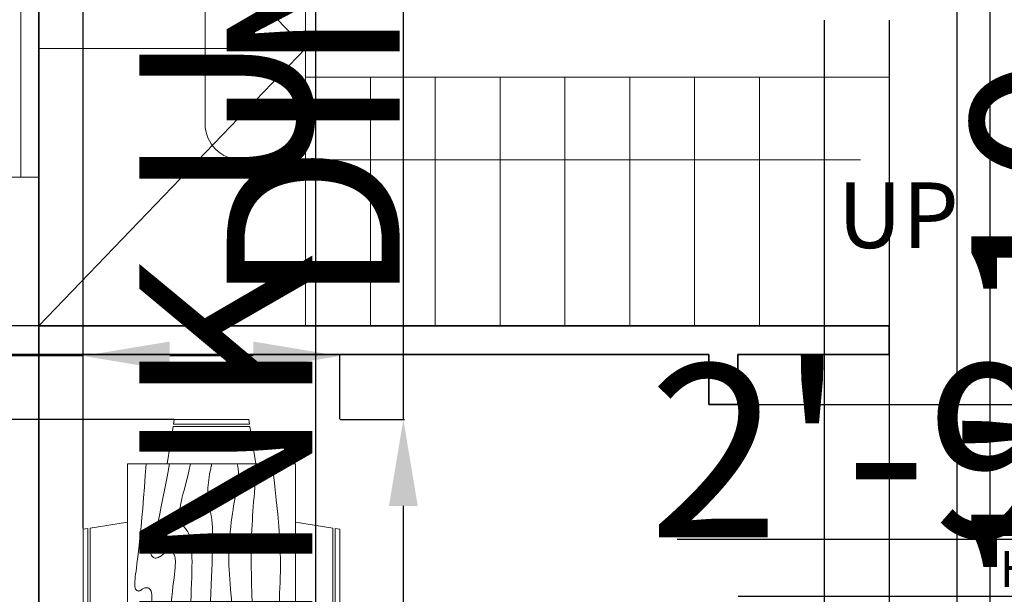
# Model space of a CAD drawing. Units: inches. Extents: x 2236 to 2927, y 1577 to 2452.
# Tile 4 of 9: x 2413 to 2550, y 1836 to 1916. Entities that reach past the tile are written whole.
import ezdxf

# ---------------------------------------------------------------- set-up
doc = ezdxf.new("R2010")
doc.units = ezdxf.units.IN
for name, color, linetype, lineweight in [('A-ANNO-DIMS', 2, 'Continuous', 18), ('A-ANNO-SYMB', 7, 'Continuous', 18), ('A-ANNO-TEXT', 7, 'Continuous', 18), ('A-AREA-IDEN', 7, 'Continuous', 18), ('A-FURN', 8, 'Continuous', 18), ('Steps', 50, 'Continuous', 18), ('Wall', 7, 'Continuous', 35), ('Windows', 162, 'Continuous', 18)]:
    doc.layers.add(name, color=color, linetype=linetype, lineweight=lineweight)
doc.styles.get("Standard").update_dxf_attribs({"font": 'arial.ttf'})
doc.dimstyles.get("Standard").update_dxf_attribs({"dimtxt": 24, "dimasz": 12, "dimexe": 0.18, "dimexo": 0.0625, "dimgap": 0.09, "dimtad": 1, "dimdec": 1, "dimzin": 0, "dimdsep": 46, "dimlunit": 4, "dimtxsty": 'Standard', "dimcen": 0.09, "dimadec": 0, "dimazin": 0, "dimtfac": 1, "dimtdec": 1, "dimtofl": 0, "dimtmove": 0, "dimatfit": 3, "dimfxl": 1, "dimtolj": 1, "dimtzin": 0, "dimarcsym": 0})

# ---------------------------------------------------------------- blocks, each defined once
blk = doc.blocks.new('Dining Set - 36 x 72 in.')
for p, q in [((-22, 27.5), (-22.1562, 26.50042)), ((-22, 27.5), (-6, 27.5)), ((-5.8437, 26.49966), (-6, 27.5)), ((6, 27.5), (5.8438, 26.50042)), ((6, 27.5), (22, 27.5)), ((22.1563, 26.49966), (22, 27.5)), ((-22.2343, 26.00059), (-23.4847, 17.99762)), ((-22.2304, 26), (-5.7608, 26)), ((-5.8416, 26.5), (-22.1534, 26.5)), ((-4.5152, 17.99762), (-5.7655, 25.99926)), ((5.7657, 26.00059), (4.5153, 17.99762)), ((5.7696, 26), (22.2392, 26)), ((22.1584, 26.5), (5.8466, 26.5)), ((23.4848, 17.99762), (22.2345, 25.99926)), ((36, 18), (-36, 18)), ((-36, 18), (-36, -18)), ((36, -18), (36, 18)), ((-44.0006, 8.23428), (-35.9976, 9.48474)), ((44.0006, 8.23428), (35.9976, 9.48474)), ((-45.5, 8), (-44.5004, 8.15617)), ((-45.5, 8), (-45.5, -8)), ((-44.5, -8.15843), (-44.5, 8.15338)), ((-44, 8.23041), (-44, -8.23915)), ((44, 8.23041), (44, -8.23915)), ((44.5, -8.15843), (44.5, 8.15338)), ((45.5, 8), (44.5005, 8.15617)), ((45.5, 8), (45.5, -8)), ((-44.4997, -8.15631), (-45.5, -8)), ((-35.9976, -9.48476), (-43.9993, -8.2345)), ((35.9976, -9.48476), (43.9993, -8.2345)), ((44.4997, -8.15631), (45.5, -8)), ((-36, -18), (36, -18)), ((-22.2343, -26.0006), (-23.4847, -17.99762)), ((-4.5152, -17.99762), (-5.7655, -25.99928)), ((5.7657, -26.0006), (4.5153, -17.99762)), ((23.4848, -17.99762), (22.2345, -25.99928)), ((-22.2304, -26), (-5.7608, -26)), ((-22, -27.5), (-22.1562, -26.50044)), ((-5.8416, -26.5), (-22.1534, -26.5)), ((-5.8437, -26.49967), (-6, -27.5)), ((5.7696, -26), (22.2392, -26)), ((6, -27.5), (5.8438, -26.50044)), ((22.1584, -26.5), (5.8466, -26.5)), ((22.1563, -26.49967), (22, -27.5)), ((-22, -27.5), (-6, -27.5)), ((6, -27.5), (22, -27.5))]:
    blk.add_line(p, q)
for points in [[(-36, 15), (-31.1772, 14.97754), (-26.8079, 14.91406), (-22.8538, 14.81543), (-19.276, 14.6875), (-16.0362, 14.53613), (-13.0957, 14.36718), (-10.4159, 14.18652), (-7.9583, 14), (-5.6904, 13.81315), (-3.6035, 13.63021), (-1.6954, 13.45508), (0.0365, 13.29166), (1.5945, 13.14388), (2.9811, 13.01562), (4.1988, 12.9108), (5.25, 12.83333), (6.1393, 12.78613), (6.8802, 12.76823), (7.4883, 12.77767), (7.9792, 12.8125), (8.3685, 12.87077), (8.6719, 12.95052), (8.9049, 13.0498), (9.0833, 13.16666), (9.2205, 13.29899), (9.3216, 13.44401), (9.3895, 13.59879), (9.4271, 13.76041), (9.4373, 13.92594), (9.4232, 14.09245), (9.3875, 14.257), (9.3333, 14.41666), (9.2638, 14.56917), (9.1836, 14.71484), (9.0975, 14.85465), (9.0104, 14.98958), (8.9272, 15.1206), (8.8529, 15.2487), (8.7922, 15.37483), (8.75, 15.5), (8.7305, 15.62467), (8.7344, 15.74739), (8.7617, 15.86621), (8.8125, 15.97916), (8.8867, 16.08431), (8.9844, 16.17968), (9.1055, 16.26334), (9.25, 16.33333), (9.4189, 16.38802), (9.6172, 16.42708), (9.8506, 16.45052), (10.125, 16.45833), (10.4463, 16.45052), (10.8203, 16.42708), (11.2529, 16.38802), (11.75, 16.33333), (12.3184, 16.26318), (12.9694, 16.17838), (13.7151, 16.07991), (14.5677, 15.96875), (15.5395, 15.84586), (16.6426, 15.71224), (17.8893, 15.56884), (19.2917, 15.41666), (20.859, 15.25667), (22.5879, 15.08984), (24.4721, 14.91715), (26.5052, 14.73958), (28.6809, 14.5581), (30.9929, 14.3737), (33.4347, 14.18733), (36, 14)], [(-36, 10), (-28.9766, 10.14274), (-23.1725, 10.20442), (-18.4241, 10.19775), (-14.5677, 10.13541), (-11.4399, 10.03011), (-8.877, 9.89453), (-6.7154, 9.74137), (-4.7917, 9.58333), (-2.9698, 9.43082), (-1.2246, 9.28515), (0.4415, 9.14534), (2.026, 9.01041), (3.5266, 8.87939), (4.9408, 8.7513), (6.266, 8.62516), (7.5, 8.5), (8.6411, 8.37549), (9.6914, 8.2539), (10.6538, 8.13818), (11.5312, 8.03125), (12.3267, 7.93603), (13.043, 7.85547), (13.6831, 7.79248), (14.25, 7.75), (14.7471, 7.7303), (15.1797, 7.73307), (15.5537, 7.75732), (15.875, 7.80208), (16.1494, 7.86637), (16.3828, 7.94922), (16.5811, 8.04964), (16.75, 8.16666), (16.8944, 8.29915), (17.0143, 8.44531), (17.1089, 8.60319), (17.1771, 8.77083), (17.218, 8.94629), (17.2305, 9.1276), (17.2137, 9.31282), (17.1667, 9.5), (17.0895, 9.6875), (16.987, 9.875), (16.8649, 10.0625), (16.7292, 10.25), (16.5856, 10.4375), (16.4401, 10.625), (16.2985, 10.8125), (16.1667, 11), (16.05, 11.18733), (15.9518, 11.3737), (15.8752, 11.5581), (15.8229, 11.73958), (15.798, 11.91715), (15.8034, 12.08984), (15.842, 12.25667), (15.9167, 12.41666), (16.0295, 12.56836), (16.1784, 12.70833), (16.3605, 12.83268), (16.5729, 12.9375), (16.8127, 13.01888), (17.0768, 13.07291), (17.3625, 13.0957), (17.6667, 13.08333), (17.9894, 13.03312), (18.3418, 12.94726), (18.7382, 12.82918), (19.1927, 12.68229), (19.7195, 12.51001), (20.3327, 12.31575), (21.0465, 12.10294), (21.875, 11.875), (22.8357, 11.63354), (23.959, 11.37304), (25.2786, 11.08618), (26.8282, 10.76562), (28.6414, 10.40405), (30.752, 9.99414), (33.1936, 9.52856), (36, 9)], [(-36, 5.5), (-30.7157, 5.3348), (-26.069, 5.20963), (-21.9946, 5.11767), (-18.4271, 5.05208), (-15.3009, 5.00602), (-12.5508, 4.97265), (-10.1112, 4.94515), (-7.9167, 4.91666), (-5.909, 4.88167), (-4.0586, 4.83984), (-2.3429, 4.79215), (-0.7396, 4.73958), (0.7739, 4.6831), (2.22, 4.6237), (3.6213, 4.56233), (5, 4.5), (6.373, 4.43782), (7.7344, 4.3776), (9.0723, 4.32129), (10.375, 4.27083), (11.6309, 4.22819), (12.8281, 4.19531), (13.9551, 4.17415), (15, 4.16666), (15.954, 4.17448), (16.819, 4.19791), (17.6001, 4.23698), (18.3021, 4.29166), (18.9299, 4.36198), (19.4883, 4.44791), (19.9823, 4.54948), (20.4167, 4.66666), (20.7969, 4.79899), (21.1302, 4.94401), (21.4245, 5.09879), (21.6875, 5.26041), (21.9271, 5.42594), (22.1511, 5.59245), (22.3672, 5.757), (22.5834, 5.91666), (22.8065, 6.06868), (23.0404, 6.21093), (23.2879, 6.34147), (23.5521, 6.45833), (23.8358, 6.55957), (24.142, 6.64323), (24.4735, 6.70735), (24.8334, 6.75), (25.2235, 6.76969), (25.642, 6.76692), (26.0858, 6.74267), (26.5521, 6.69791), (27.0379, 6.63362), (27.5404, 6.55078), (28.0565, 6.45036), (28.5834, 6.33333), (29.1242, 6.19987), (29.7071, 6.04687), (30.3661, 5.87044), (31.1354, 5.66666), (32.0493, 5.43164), (33.142, 5.16146), (34.4475, 4.85221), (36, 4.5)], [(-36, -1), (-30.7915, -0.6591), (-26.0195, -0.38216), (-21.6519, -0.16284), (-17.6563, 0.00521), (-14.0005, 0.12833), (-10.6523, 0.21289), (-7.5796, 0.26522), (-4.75, 0.29166), (-2.134, 0.29793), (0.2878, 0.28711), (2.5317, 0.26163), (4.6146, 0.22396), (6.5529, 0.17651), (8.3633, 0.12174), (10.0623, 0.06209), (11.6667, 0), (13.1899, -0.06201), (14.6341, -0.1211), (15.9982, -0.17432), (17.2813, -0.21875), (18.4823, -0.25147), (19.6003, -0.26953), (20.6343, -0.27002), (21.5834, -0.25), (22.4481, -0.20768), (23.2357, -0.14584), (23.9549, -0.06836), (24.6146, 0.02083), (25.2235, 0.11784), (25.7904, 0.21875), (26.3241, 0.31966), (26.8334, 0.41666), (27.3265, 0.50618), (27.8099, 0.58593), (28.2894, 0.65397), (28.7709, 0.70833), (29.2601, 0.74707), (29.763, 0.76823), (30.2855, 0.76985), (30.8334, 0.75), (31.4088, 0.70784), (31.9994, 0.64713), (32.589, 0.57275), (33.1615, 0.48958), (33.7008, 0.4025), (34.1908, 0.3164), (34.6153, 0.23616), (34.9584, 0.16666), (35.2099, 0.11165), (35.3848, 0.07031), (35.504, 0.04069), (35.5886, 0.02083), (35.6594, 0.00879), (35.7377, 0.0026), (35.8442, 0.00032), (36, 0)], [(-36, -6.5), (-27.1843, -6.31267), (-20.084, -6.1263), (-14.469, -5.9419), (-10.1094, -5.76042), (-6.7752, -5.58285), (-4.2363, -5.41016), (-2.2629, -5.24333), (-0.625, -5.08334), (0.8708, -4.93099), (2.2715, -4.78646), (3.5872, -4.64974), (4.8281, -4.52084), (6.0046, -4.39974), (7.127, -4.28646), (8.2053, -4.18099), (9.25, -4.08334), (10.2705, -3.99382), (11.2734, -3.91407), (12.2647, -3.84603), (13.25, -3.79167), (14.2354, -3.75293), (15.2266, -3.73177), (16.2295, -3.73015), (17.25, -3.75), (18.2912, -3.79248), (19.3451, -3.85547), (20.4009, -3.93604), (21.4479, -4.03125), (22.4754, -4.13819), (23.4727, -4.25391), (24.4289, -4.37549), (25.3334, -4.5), (26.1785, -4.62492), (26.9694, -4.74935), (27.7145, -4.87281), (28.4219, -4.99479), (29.1, -5.11483), (29.7572, -5.23242), (30.4016, -5.34709), (31.0417, -5.45834), (31.6837, -5.56437), (32.3262, -5.65821), (32.9658, -5.73153), (33.599, -5.77604), (34.2224, -5.78345), (34.8327, -5.74545), (35.4264, -5.65373), (36, -5.5)], [(-36, -10), (-26.4022, -9.81299), (-18.4675, -9.62891), (-11.9839, -9.45069), (-6.7396, -9.28125), (-2.5226, -9.12354), (0.8789, -8.98047), (3.6769, -8.85498), (6.0833, -8.75), (8.2767, -8.66765), (10.3021, -8.60677), (12.1712, -8.56543), (13.8958, -8.54167), (15.4876, -8.53353), (16.9583, -8.53907), (18.3197, -8.55632), (19.5834, -8.58334), (20.7616, -8.61841), (21.8685, -8.66081), (22.9188, -8.71004), (23.9271, -8.76563), (24.9081, -8.82707), (25.8763, -8.89388), (26.8465, -8.96558), (27.8334, -9.04167), (28.8474, -9.12118), (29.8828, -9.20117), (30.93, -9.27824), (31.9792, -9.34896), (33.0205, -9.40991), (34.0443, -9.45768), (35.0407, -9.48885), (36, -9.5)], [(-36, -14.5), (-30.0881, -14.33513), (-25.0332, -14.21224), (-20.7312, -14.12647), (-17.0781, -14.07292), (-13.97, -14.04671), (-11.3027, -14.04297), (-8.9724, -14.05681), (-6.875, -14.08334), (-4.9224, -14.11833), (-3.0905, -14.16016), (-1.3709, -14.20785), (0.2448, -14.26042), (1.7647, -14.3169), (3.1973, -14.3763), (4.5507, -14.43767), (5.8333, -14.5), (7.0554, -14.5621), (8.235, -14.62175), (9.3922, -14.67652), (10.5469, -14.72396), (11.7192, -14.76164), (12.929, -14.78711), (14.1965, -14.79794), (15.5417, -14.79167), (16.9933, -14.76424), (18.6152, -14.70508), (20.4804, -14.60197), (22.6615, -14.44271), (25.2312, -14.21509), (28.2624, -13.9069), (31.8277, -13.50594), (36, -13)]]:
    blk.add_lwpolyline(points)
blk = doc.blocks.new('WIN-36IN')
for p, q in [((2.5, 0), (2.5, 36)), ((4.5, 0), (4.5, 36)), ((6.5, 0), (6.5, 36))]:
    blk.add_line(p, q)
blk.add_lwpolyline([(0, 0), (0, 36), (9, 36), (9, 0)], close=True)
blk = doc.blocks.new('*D18')
at = {"layer": 'A-ANNO-DIMS', "color": 0, "lineweight": -2, "transparency": 16777216}
for p, q in [((2396.05, 1834.44), (2396.05, 2191.28)), ((2406.79, 1834.44), (2395.87, 1834.44)), ((2396.05, 1774.44), (2396.05, 1822.44)), ((2406.79, 1762.44), (2395.87, 1762.44))]:
    blk.add_line(p, q, dxfattribs=at)
at = {"layer": 'A-ANNO-DIMS', "color": 0, "transparency": 16777216}
for points in [[(2394.05, 1822.44), (2398.05, 1822.44), (2396.05, 1834.44)], [(2394.05, 1774.44), (2398.05, 1774.44), (2396.05, 1762.44)]]:
    blk.add_solid(points, dxfattribs=at)
at = {"layer": 'Defpoints', "color": 0, "transparency": 16777216}
for p in [(2396.05, 1834.44), (2406.85, 1834.44), (2406.85, 1762.44)]:
    blk.add_point(p, dxfattribs=at)
at = {"layer": 'A-ANNO-DIMS', "color": 0, "transparency": 16777216, "insert": (2383.54, 2018.86), "char_height": 24, "attachment_point": 5, "rotation": 90}
blk.add_mtext('\\A1;WINDOW W 6\'-0" TYP.', dxfattribs=at)
blk = doc.blocks.new('*D20')
at = {"layer": 'A-ANNO-DIMS', "color": 0, "lineweight": -2, "transparency": 16777216}
for p, q in [((2401.45, 1929.71), (2401.45, 2363.75)), ((2406.79, 1929.71), (2401.27, 1929.71)), ((2401.45, 1905.71), (2401.45, 1917.71)), ((2406.79, 1893.71), (2401.27, 1893.71))]:
    blk.add_line(p, q, dxfattribs=at)
at = {"layer": 'A-ANNO-DIMS', "color": 0, "transparency": 16777216}
for points in [[(2399.45, 1917.71), (2403.45, 1917.71), (2401.45, 1929.71)], [(2399.45, 1905.71), (2403.45, 1905.71), (2401.45, 1893.71)]]:
    blk.add_solid(points, dxfattribs=at)
at = {"layer": 'Defpoints', "color": 0, "transparency": 16777216}
for p in [(2401.45, 1929.71), (2406.85, 1929.71), (2406.85, 1893.71)]:
    blk.add_point(p, dxfattribs=at)
at = {"layer": 'A-ANNO-DIMS', "color": 0, "transparency": 16777216, "insert": (2388.93, 2152.73), "char_height": 24, "attachment_point": 5, "rotation": 90}
blk.add_mtext('\\A1;SMALL WINDOW 3\'-0" TYP.', dxfattribs=at)
blk = doc.blocks.new('*D21')
at = {"layer": 'A-ANNO-DIMS', "color": 0, "lineweight": -2, "transparency": 16777216}
for p, q in [((2394.85, 1935.11), (2382.85, 1935.11)), ((2406.85, 1929.77), (2406.85, 1935.29)), ((2415.85, 1929.77), (2415.85, 1935.29)), ((2427.85, 1935.11), (2586.32, 1935.11))]:
    blk.add_line(p, q, dxfattribs=at)
at = {"layer": 'A-ANNO-DIMS', "color": 0, "transparency": 16777216}
for points in [[(2394.85, 1937.11), (2394.85, 1933.11), (2406.85, 1935.11)], [(2427.85, 1937.11), (2427.85, 1933.11), (2415.85, 1935.11)]]:
    blk.add_solid(points, dxfattribs=at)
at = {"layer": 'Defpoints', "color": 0, "transparency": 16777216}
for p in [(2415.85, 1935.11), (2406.85, 1929.71), (2415.85, 1929.71)]:
    blk.add_point(p, dxfattribs=at)
at = {"layer": 'A-ANNO-DIMS', "color": 0, "transparency": 16777216, "insert": (2513.08, 1947.45), "char_height": 24, "attachment_point": 5}
blk.add_mtext('\\A1;0\'-9" TYP.', dxfattribs=at)
blk = doc.blocks.new('*D23')
at = {"layer": 'A-ANNO-DIMS', "color": 0, "lineweight": -2, "transparency": 16777216}
for p, q in [((2518.6, 1950.01), (2518.6, 1945.71)), ((2543.24, 1950.01), (2543.24, 1945.71)), ((2518.6, 1945.89), (2303.79, 1945.89)), ((2531.24, 1945.89), (2530.6, 1945.89))]:
    blk.add_line(p, q, dxfattribs=at)
at = {"layer": 'A-ANNO-DIMS', "color": 0, "transparency": 16777216}
for points in [[(2530.6, 1947.89), (2530.6, 1943.89), (2518.6, 1945.89)], [(2531.24, 1947.89), (2531.24, 1943.89), (2543.24, 1945.89)]]:
    blk.add_solid(points, dxfattribs=at)
at = {"layer": 'Defpoints', "color": 0, "transparency": 16777216}
for p in [(2518.6, 1950.08), (2543.24, 1950.08), (2518.6, 1945.89)]:
    blk.add_point(p, dxfattribs=at)
at = {"layer": 'A-ANNO-DIMS', "color": 0, "transparency": 16777216, "insert": (2405.19, 1958.39), "char_height": 24, "attachment_point": 5}
blk.add_mtext('\\A1;2\'-0 1/2" TYP.', dxfattribs=at)
blk = doc.blocks.new('*D33')
at = {"layer": 'A-ANNO-DIMS', "color": 0, "lineweight": -2, "transparency": 16777216}
for p, q in [((2580.85, 1855.01), (2580.85, 1843.2)), ((2613.85, 1855.01), (2613.85, 1843.2)), ((2580.85, 1843.38), (2504.46, 1843.38)), ((2601.85, 1843.38), (2592.85, 1843.38))]:
    blk.add_line(p, q, dxfattribs=at)
at = {"layer": 'A-ANNO-DIMS', "color": 0, "transparency": 16777216}
for points in [[(2592.85, 1845.38), (2592.85, 1841.38), (2580.85, 1843.38)], [(2601.85, 1845.38), (2601.85, 1841.38), (2613.85, 1843.38)]]:
    blk.add_solid(points, dxfattribs=at)
at = {"layer": 'Defpoints', "color": 0, "transparency": 16777216}
for p in [(2580.85, 1855.08), (2613.85, 1855.08), (2580.85, 1843.38)]:
    blk.add_point(p, dxfattribs=at)
at = {"layer": 'A-ANNO-DIMS', "color": 0, "transparency": 16777216, "insert": (2536.65, 1855.72), "char_height": 24, "attachment_point": 5}
blk.add_mtext('\\A1;2\'-9"', dxfattribs=at)
blk = doc.blocks.new('*D34')
at = {"layer": 'A-ANNO-DIMS', "color": 0, "lineweight": -2, "transparency": 16777216}
for p, q in [((2520.69, 1794.44), (2520.69, 1787.92)), ((2563.35, 1794.44), (2563.35, 1787.92)), ((2532.69, 1788.1), (2551.35, 1788.1)), ((2563.35, 1788.1), (2926.83, 1788.1))]:
    blk.add_line(p, q, dxfattribs=at)
at = {"layer": 'A-ANNO-DIMS', "color": 0, "transparency": 16777216}
for points in [[(2532.69, 1790.1), (2532.69, 1786.1), (2520.69, 1788.1)], [(2551.35, 1790.1), (2551.35, 1786.1), (2563.35, 1788.1)]]:
    blk.add_solid(points, dxfattribs=at)
at = {"layer": 'Defpoints', "color": 0, "transparency": 16777216}
for p in [(2520.69, 1794.5), (2563.35, 1794.5), (2563.35, 1788.1)]:
    blk.add_point(p, dxfattribs=at)
at = {"layer": 'A-ANNO-DIMS', "color": 0, "transparency": 16777216, "insert": (2751.09, 1800.62), "char_height": 24, "attachment_point": 5}
blk.add_mtext('\\A1;ENTRY DOOR 3\'-6 1/2"', dxfattribs=at)
blk = doc.blocks.new('*D35')
at = {"layer": 'A-ANNO-DIMS', "color": 0, "lineweight": -2, "transparency": 16777216}
for p, q in [((2569.75, 1828.98), (2569.75, 1977.27)), ((2563.41, 1816.98), (2569.93, 1816.98)), ((2563.41, 1794.5), (2569.93, 1794.5)), ((2569.75, 1782.5), (2569.75, 1770.5))]:
    blk.add_line(p, q, dxfattribs=at)
at = {"layer": 'A-ANNO-DIMS', "color": 0, "transparency": 16777216}
for points in [[(2567.75, 1828.98), (2571.75, 1828.98), (2569.75, 1816.98)], [(2567.75, 1782.5), (2571.75, 1782.5), (2569.75, 1794.5)]]:
    blk.add_solid(points, dxfattribs=at)
at = {"layer": 'Defpoints', "color": 0, "transparency": 16777216}
for p in [(2563.35, 1816.98), (2569.75, 1816.98), (2563.35, 1794.5)]:
    blk.add_point(p, dxfattribs=at)
at = {"layer": 'A-ANNO-DIMS', "color": 0, "transparency": 16777216, "insert": (2557.25, 1909.13), "char_height": 24, "attachment_point": 5, "rotation": 90}
blk.add_mtext('\\A1;1\'-10 1/2"', dxfattribs=at)
blk = doc.blocks.new('*D36')
at = {"layer": 'A-ANNO-DIMS', "color": 0, "lineweight": -2, "transparency": 16777216}
for p, q in [((2454.3, 1796.23), (2454.3, 2047.2)), ((2444.91, 1796.23), (2454.48, 1796.23)), ((2454.3, 1745.23), (2454.3, 1784.23)), ((2444.91, 1733.23), (2454.48, 1733.23))]:
    blk.add_line(p, q, dxfattribs=at)
at = {"layer": 'A-ANNO-DIMS', "color": 0, "transparency": 16777216}
for points in [[(2452.3, 1784.23), (2456.3, 1784.23), (2454.3, 1796.23)], [(2452.3, 1745.23), (2456.3, 1745.23), (2454.3, 1733.23)]]:
    blk.add_solid(points, dxfattribs=at)
at = {"layer": 'Defpoints', "color": 0, "transparency": 16777216}
for p in [(2444.85, 1796.23), (2454.3, 1796.23), (2444.85, 1733.23)]:
    blk.add_point(p, dxfattribs=at)
at = {"layer": 'A-ANNO-DIMS', "color": 0, "transparency": 16777216, "insert": (2441.79, 1927.72), "char_height": 24, "attachment_point": 5, "rotation": 90}
blk.add_mtext('\\A1;SINK UNIT 5\'-3"', dxfattribs=at)
blk = doc.blocks.new('*D38')
at = {"layer": 'A-ANNO-DIMS', "color": 0, "lineweight": -2, "transparency": 16777216}
for p, q in [((2466.44, 1860.06), (2466.44, 2154.67)), ((2457.67, 1860.06), (2466.62, 1860.06)), ((2466.44, 1813.15), (2466.44, 1848.06)), ((2457.67, 1801.15), (2466.62, 1801.15))]:
    blk.add_line(p, q, dxfattribs=at)
at = {"layer": 'A-ANNO-DIMS', "color": 0, "transparency": 16777216}
for points in [[(2464.44, 1848.06), (2468.44, 1848.06), (2466.44, 1860.06)], [(2464.44, 1813.15), (2468.44, 1813.15), (2466.44, 1801.15)]]:
    blk.add_solid(points, dxfattribs=at)
at = {"layer": 'Defpoints', "color": 0, "transparency": 16777216}
for p in [(2457.61, 1860.06), (2466.44, 1860.06), (2457.61, 1801.15)]:
    blk.add_point(p, dxfattribs=at)
at = {"layer": 'A-ANNO-DIMS', "color": 0, "transparency": 16777216, "insert": (2453.94, 2013.36), "char_height": 24, "attachment_point": 5, "rotation": 90}
blk.add_mtext('\\A1;DINING SET 4\'-11"', dxfattribs=at)
blk = doc.blocks.new('*D39')
at = {"layer": 'A-ANNO-DIMS', "color": 0, "lineweight": -2, "transparency": 16777216}
for p, q in [((2422.01, 1868.89), (2271.05, 1868.89)), ((2422.01, 1860.12), (2422.01, 1869.07)), ((2445.61, 1868.89), (2434.01, 1868.89)), ((2457.61, 1860.12), (2457.61, 1869.07))]:
    blk.add_line(p, q, dxfattribs=at)
at = {"layer": 'A-ANNO-DIMS', "color": 0, "transparency": 16777216}
for points in [[(2434.01, 1870.89), (2434.01, 1866.89), (2422.01, 1868.89)], [(2445.61, 1870.89), (2445.61, 1866.89), (2457.61, 1868.89)]]:
    blk.add_solid(points, dxfattribs=at)
at = {"layer": 'Defpoints', "color": 0, "transparency": 16777216}
for p in [(2422.01, 1868.89), (2422.01, 1860.06), (2457.61, 1860.06)]:
    blk.add_point(p, dxfattribs=at)
at = {"layer": 'A-ANNO-DIMS', "color": 0, "transparency": 16777216, "insert": (2340.53, 1881.39), "char_height": 24, "attachment_point": 5}
blk.add_mtext('\\A1;2\'-11 1/2"', dxfattribs=at)
blk = doc.blocks.new('*D46')
at = {"layer": 'A-ANNO-DIMS', "color": 0, "lineweight": -2, "transparency": 16777216}
for p, q in [((2415.85, 1873.01), (2415.85, 1702.15)), ((2533.86, 1873.01), (2533.86, 1702.15)), ((2427.85, 1702.33), (2521.86, 1702.33))]:
    blk.add_line(p, q, dxfattribs=at)
at = {"layer": 'A-ANNO-DIMS', "color": 0, "transparency": 16777216}
for points in [[(2427.85, 1704.33), (2427.85, 1700.33), (2415.85, 1702.33)], [(2521.86, 1704.33), (2521.86, 1700.33), (2533.86, 1702.33)]]:
    blk.add_solid(points, dxfattribs=at)
at = {"layer": 'Defpoints', "color": 0, "transparency": 16777216}
for p in [(2415.85, 1873.08), (2533.86, 1873.08), (2533.86, 1702.33)]:
    blk.add_point(p, dxfattribs=at)
at = {"layer": 'A-ANNO-DIMS', "color": 0, "transparency": 16777216, "insert": (2474.85, 1714.67), "char_height": 24, "attachment_point": 5}
blk.add_mtext('\\A1;9\'-10"', dxfattribs=at)
blk = doc.blocks.new('*D47')
at = {"layer": 'A-ANNO-DIMS', "color": 0, "lineweight": -2, "transparency": 16777216}
for p, q in [((2415.79, 1950.08), (2384.92, 1950.08)), ((2385.1, 1885.08), (2385.1, 1938.08)), ((2415.79, 1873.08), (2384.92, 1873.08))]:
    blk.add_line(p, q, dxfattribs=at)
at = {"layer": 'A-ANNO-DIMS', "color": 0, "transparency": 16777216}
for points in [[(2383.1, 1938.08), (2387.1, 1938.08), (2385.1, 1950.08)], [(2383.1, 1885.08), (2387.1, 1885.08), (2385.1, 1873.08)]]:
    blk.add_solid(points, dxfattribs=at)
at = {"layer": 'Defpoints', "color": 0, "transparency": 16777216}
for p in [(2385.1, 1950.08), (2415.85, 1950.08), (2415.85, 1873.08)]:
    blk.add_point(p, dxfattribs=at)
at = {"layer": 'A-ANNO-DIMS', "color": 0, "transparency": 16777216, "insert": (2372.75, 1911.58), "char_height": 24, "attachment_point": 5, "rotation": 90}
blk.add_mtext('\\A1;6\'-5"', dxfattribs=at)
blk = doc.blocks.new('*D48')
at = {"layer": 'A-ANNO-DIMS', "color": 0, "lineweight": -2, "transparency": 16777216}
for p, q in [((2524.86, 1915.51), (2524.86, 1702.15)), ((2533.86, 1915.51), (2533.86, 1702.15)), ((2512.86, 1702.33), (2500.86, 1702.33)), ((2545.86, 1702.33), (2621.84, 1702.33))]:
    blk.add_line(p, q, dxfattribs=at)
at = {"layer": 'A-ANNO-DIMS', "color": 0, "transparency": 16777216}
for points in [[(2512.86, 1704.33), (2512.86, 1700.33), (2524.86, 1702.33)], [(2545.86, 1704.33), (2545.86, 1700.33), (2533.86, 1702.33)]]:
    blk.add_solid(points, dxfattribs=at)
at = {"layer": 'Defpoints', "color": 0, "transparency": 16777216}
for p in [(2524.86, 1915.58), (2533.86, 1915.58), (2533.86, 1702.33)]:
    blk.add_point(p, dxfattribs=at)
at = {"layer": 'A-ANNO-DIMS', "color": 0, "transparency": 16777216, "insert": (2589.85, 1714.67), "char_height": 24, "attachment_point": 5}
blk.add_mtext('\\A1;0\'-9"', dxfattribs=at)
blk = doc.blocks.new('*D51')
at = {"layer": 'A-ANNO-DIMS', "color": 0, "lineweight": -2, "transparency": 16777216}
for p, q in [((2644.6, 1862.15), (2644.6, 1994.46)), ((2512.91, 1862.15), (2644.78, 1862.15)), ((2644.6, 1847.53), (2644.6, 1850.15)), ((2512.91, 1835.53), (2644.78, 1835.53))]:
    blk.add_line(p, q, dxfattribs=at)
at = {"layer": 'A-ANNO-DIMS', "color": 0, "transparency": 16777216}
for points in [[(2642.6, 1850.15), (2646.6, 1850.15), (2644.6, 1862.15)], [(2642.6, 1847.53), (2646.6, 1847.53), (2644.6, 1835.53)]]:
    blk.add_solid(points, dxfattribs=at)
at = {"layer": 'Defpoints', "color": 0, "transparency": 16777216}
for p in [(2512.85, 1862.15), (2644.6, 1862.15), (2512.85, 1835.53)]:
    blk.add_point(p, dxfattribs=at)
at = {"layer": 'A-ANNO-DIMS', "color": 0, "transparency": 16777216, "insert": (2632.1, 1934.31), "char_height": 24, "attachment_point": 5, "rotation": 90}
blk.add_mtext('\\A1;2\'-2 1/2"', dxfattribs=at)
blk = doc.blocks.new('*D54')
at = {"layer": 'A-ANNO-DIMS', "color": 0, "lineweight": -2, "transparency": 16777216}
for p, q in [((2543.24, 1954.99), (2543.24, 1702.15)), ((2547.85, 1955.01), (2547.85, 1702.15)), ((2531.24, 1702.33), (2519.24, 1702.33)), ((2559.85, 1702.33), (2691.75, 1702.33))]:
    blk.add_line(p, q, dxfattribs=at)
at = {"layer": 'A-ANNO-DIMS', "color": 0, "transparency": 16777216}
for points in [[(2531.24, 1704.33), (2531.24, 1700.33), (2543.24, 1702.33)], [(2559.85, 1704.33), (2559.85, 1700.33), (2547.85, 1702.33)]]:
    blk.add_solid(points, dxfattribs=at)
at = {"layer": 'Defpoints', "color": 0, "transparency": 16777216}
for p in [(2543.24, 1955.06), (2547.85, 1955.08), (2547.85, 1702.33)]:
    blk.add_point(p, dxfattribs=at)
at = {"layer": 'A-ANNO-DIMS', "color": 0, "transparency": 16777216, "insert": (2631.8, 1714.83), "char_height": 24, "attachment_point": 5}
blk.add_mtext('\\A1;0\'-4 1/2"', dxfattribs=at)
blk = doc.blocks.new('*D56')
at = {"layer": 'A-ANNO-DIMS', "color": 0, "lineweight": -2, "transparency": 16777216}
for p, q in [((2551.88, 1874.28), (2551.88, 1702.15)), ((2569.42, 1874.28), (2569.42, 1702.15)), ((2539.88, 1702.33), (2527.88, 1702.33)), ((2581.42, 1702.33), (2711.06, 1702.33))]:
    blk.add_line(p, q, dxfattribs=at)
at = {"layer": 'A-ANNO-DIMS', "color": 0, "transparency": 16777216}
for points in [[(2539.88, 1704.33), (2539.88, 1700.33), (2551.88, 1702.33)], [(2581.42, 1704.33), (2581.42, 1700.33), (2569.42, 1702.33)]]:
    blk.add_solid(points, dxfattribs=at)
at = {"layer": 'Defpoints', "color": 0, "transparency": 16777216}
for p in [(2551.88, 1874.34), (2569.42, 1874.34), (2569.42, 1702.33)]:
    blk.add_point(p, dxfattribs=at)
at = {"layer": 'A-ANNO-DIMS', "color": 0, "transparency": 16777216, "insert": (2652.24, 1714.83), "char_height": 24, "attachment_point": 5}
blk.add_mtext('\\A1;1\'-5 1/2"', dxfattribs=at)
blk = doc.blocks.new('*D60')
at = {"layer": 'A-ANNO-DIMS', "color": 0, "lineweight": -2, "transparency": 16777216}
for p, q in [((2385.1, 1881.08), (2385.1, 1957.05)), ((2415.79, 1869.08), (2384.92, 1869.08)), ((2434.57, 1860.06), (2384.92, 1860.06)), ((2385.1, 1848.06), (2385.1, 1836.06))]:
    blk.add_line(p, q, dxfattribs=at)
at = {"layer": 'A-ANNO-DIMS', "color": 0, "transparency": 16777216}
for points in [[(2383.1, 1881.08), (2387.1, 1881.08), (2385.1, 1869.08)], [(2383.1, 1848.06), (2387.1, 1848.06), (2385.1, 1860.06)]]:
    blk.add_solid(points, dxfattribs=at)
at = {"layer": 'Defpoints', "color": 0, "transparency": 16777216}
for p in [(2385.1, 1869.08), (2415.85, 1869.08), (2434.63, 1860.06)]:
    blk.add_point(p, dxfattribs=at)
at = {"layer": 'A-ANNO-DIMS', "color": 0, "transparency": 16777216, "insert": (2372.75, 1925.07), "char_height": 24, "attachment_point": 5, "rotation": 90}
blk.add_mtext('\\A1;0\'-9"', dxfattribs=at)
blk = doc.blocks.new('*D61')
at = {"layer": 'A-ANNO-DIMS', "color": 0, "lineweight": -2, "transparency": 16777216}
for p, q in [((2415.85, 1869.14), (2415.85, 2106.01)), ((2422.01, 1844.91), (2422.01, 2106.01)), ((2403.85, 2105.83), (2327.87, 2105.83)), ((2434.01, 2105.83), (2446.01, 2105.83))]:
    blk.add_line(p, q, dxfattribs=at)
at = {"layer": 'A-ANNO-DIMS', "color": 0, "transparency": 16777216}
for points in [[(2403.85, 2107.83), (2403.85, 2103.83), (2415.85, 2105.83)], [(2434.01, 2107.83), (2434.01, 2103.83), (2422.01, 2105.83)]]:
    blk.add_solid(points, dxfattribs=at)
at = {"layer": 'Defpoints', "color": 0, "transparency": 16777216}
for p in [(2415.85, 2105.83), (2415.85, 1869.08), (2422.01, 1844.84)]:
    blk.add_point(p, dxfattribs=at)
at = {"layer": 'A-ANNO-DIMS', "color": 0, "transparency": 16777216, "insert": (2359.86, 2118.17), "char_height": 24, "attachment_point": 5}
blk.add_mtext('\\A1;0\'-6"', dxfattribs=at)
blk = doc.blocks.new('*D64')
at = {"layer": 'A-ANNO-DIMS', "color": 0, "lineweight": -2, "transparency": 16777216}
for p, q in [((2569.42, 1874.28), (2569.42, 1702.15)), ((2580.85, 1860.01), (2580.85, 1702.15)), ((2557.42, 1702.33), (2545.42, 1702.33)), ((2592.85, 1702.33), (2743.4, 1702.33))]:
    blk.add_line(p, q, dxfattribs=at)
at = {"layer": 'A-ANNO-DIMS', "color": 0, "transparency": 16777216}
for points in [[(2557.42, 1704.33), (2557.42, 1700.33), (2569.42, 1702.33)], [(2592.85, 1704.33), (2592.85, 1700.33), (2580.85, 1702.33)]]:
    blk.add_solid(points, dxfattribs=at)
at = {"layer": 'Defpoints', "color": 0, "transparency": 16777216}
for p in [(2569.42, 1874.34), (2580.85, 1860.08), (2580.85, 1702.33)]:
    blk.add_point(p, dxfattribs=at)
at = {"layer": 'A-ANNO-DIMS', "color": 0, "transparency": 16777216, "insert": (2674.12, 1714.83), "char_height": 24, "attachment_point": 5}
blk.add_mtext('\\A1;0\'-11 1/2"', dxfattribs=at)

msp = doc.modelspace()

# ---------------------------------------------------------------- linework, layer by layer
at = {"layer": 'A-ANNO-SYMB'}
for p, q in [((2438.92, 1901.13), (2438.92, 1918.31)), ((2529.89, 1896.13), (2443.92, 1896.13))]:
    msp.add_line(p, q, dxfattribs=at)
msp.add_arc((2443.92, 1901.13), 5, 180, 270, dxfattribs=at)
at = {"layer": 'Steps'}
for p, q in [((2452.86, 1911.58), (2415.85, 1950.08)), ((2452.86, 1873.08), (2452.86, 1950.08)), ((2452.86, 1911.58), (2415.85, 1911.58)), ((2452.86, 1911.58), (2415.85, 1873.08)), ((2533.86, 1907.58), (2452.86, 1907.58)), ((2461.86, 1873.08), (2461.86, 1907.58)), ((2470.86, 1873.08), (2470.86, 1907.58)), ((2479.86, 1873.08), (2479.86, 1907.58)), ((2488.86, 1873.08), (2488.86, 1907.58)), ((2497.86, 1873.08), (2497.86, 1907.58)), ((2506.86, 1873.08), (2506.86, 1907.58)), ((2515.86, 1873.08), (2515.86, 1907.58)), ((2524.86, 1873.08), (2524.86, 1907.58)), ((2533.86, 1873.08), (2533.86, 1907.58))]:
    msp.add_line(p, q, dxfattribs=at)
at = {"layer": 'Wall'}
for p, q in [((2415.85, 1950.08), (2415.85, 1873.08)), ((2415.85, 1873.08), (2533.86, 1873.08)), ((2533.86, 1873.08), (2533.86, 1869.08)), ((2415.85, 1869.08), (2508.85, 1869.08)), ((2415.85, 1869.08), (2415.85, 1733.08)), ((2508.85, 1869.08), (2508.85, 1862.15)), ((2512.85, 1869.08), (2512.85, 1862.15)), ((2512.85, 1869.08), (2533.86, 1869.08)), ((2508.85, 1862.15), (2512.85, 1862.15))]:
    msp.add_line(p, q, dxfattribs=at)

# ---------------------------------------------------------------- block references
at = {"layer": 'A-FURN', "xscale": 0.6472934063691596, "yscale": 0.6472934063691596, "zscale": 0.6472934063691596, "rotation": 90}
msp.add_blockref('Dining Set - 36 x 72 in.', (2439.81, 1830.6), dxfattribs=at)
at = {"layer": 'Windows'}
msp.add_blockref('WIN-36IN', (2406.85, 1893.71), dxfattribs=at)

# ---------------------------------------------------------------- texts
at = {"layer": 'A-ANNO-TEXT'}
msp.add_text('UP', height=9.116, dxfattribs=at).set_placement((2526.7, 1883.87))
at = {"layer": 'A-AREA-IDEN', "insert": (2538.73, 1841.81), "char_height": 5, "attachment_point": 1}
msp.add_mtext_dynamic_manual_height_columns("\\pxqc;HALL\\P8'5''X15'5'", width=37.4353, gutter_width=12.5, heights=[0], dxfattribs=at)

# ---------------------------------------------------------------- dimensions: what is measured, and where the dimension line sits
at = {"layer": 'A-ANNO-DIMS'}
for base, p1, p2, angle, text, picture, middle in [((2401.45, 1929.71), (2406.85, 1893.71), (2406.85, 1929.71), 90, 'SMALL WINDOW <> TYP.', '*D20', (2388.93, 2152.73)), ((2396.05, 1834.44), (2406.85, 1762.44), (2406.85, 1834.44), 90, 'WINDOW W <> TYP.', '*D18', (2383.54, 2018.86)), ((2466.44, 1860.06), (2457.61, 1801.15), (2457.61, 1860.06), 90, 'DINING SET <>', '*D38', (2453.94, 2013.36)), ((2454.3, 1796.23), (2444.85, 1733.23), (2444.85, 1796.23), 90, 'SINK UNIT <>', '*D36', (2441.79, 1927.72)), ((2518.6, 1945.89), (2543.24, 1950.08), (2518.6, 1950.08), 180, '<> TYP.', '*D23', (2405.19, 1958.39))]:
    dim = msp.add_linear_dim(base=base, p1=p1, p2=p2, angle=angle, text=text, dimstyle='Standard', override={"dimdec": 1, "dimlfac": 1, "dimrnd": 0, "dimzin": 1, "dimdsep": 46, "dimlunit": 4, "dimfrac": 2}, dxfattribs=at)
    dim.commit()
    dim.dimension.update_dxf_attribs({"geometry": picture, "text_midpoint": middle})
for base, p1, p2, picture, middle in [((2415.85, 2105.83), (2422.01, 1844.84), (2415.85, 1869.08), '*D61', (2359.86, 2118.17)), ((2547.85, 1702.33), (2543.24, 1955.06), (2547.85, 1955.08), '*D54', (2631.8, 1714.83)), ((2533.86, 1702.33), (2524.86, 1915.58), (2533.86, 1915.58), '*D48', (2589.85, 1714.67)), ((2569.42, 1702.33), (2551.88, 1874.34), (2569.42, 1874.34), '*D56', (2652.24, 1714.83)), ((2580.85, 1702.33), (2569.42, 1874.34), (2580.85, 1860.08), '*D64', (2674.12, 1714.83)), ((2533.86, 1702.33), (2415.85, 1873.08), (2533.86, 1873.08), '*D46', (2474.85, 1714.67))]:
    dim = msp.add_linear_dim(base=base, p1=p1, p2=p2, dimstyle='Standard', override={"dimdec": 1, "dimlfac": 1, "dimrnd": 0, "dimzin": 1, "dimdsep": 46, "dimlunit": 4, "dimfrac": 2}, dxfattribs=at)
    dim.commit()
    dim.dimension.update_dxf_attribs({"geometry": picture, "text_midpoint": middle})
for base, p1, p2, angle, picture, middle in [((2644.6, 1862.15), (2512.85, 1835.53), (2512.85, 1862.15), 90, '*D51', (2632.1, 1934.31)), ((2569.75, 1816.98), (2563.35, 1794.5), (2563.35, 1816.98), 90, '*D35', (2557.25, 1909.13)), ((2385.1, 1869.08), (2434.63, 1860.06), (2415.85, 1869.08), 90, '*D60', (2372.75, 1925.07)), ((2385.1, 1950.08), (2415.85, 1873.08), (2415.85, 1950.08), 90, '*D47', (2372.75, 1911.58)), ((2422.01, 1868.89), (2457.61, 1860.06), (2422.01, 1860.06), 180, '*D39', (2340.53, 1881.39)), ((2580.85, 1843.38), (2613.85, 1855.08), (2580.85, 1855.08), 180, '*D33', (2536.65, 1855.72))]:
    dim = msp.add_linear_dim(base=base, p1=p1, p2=p2, angle=angle, dimstyle='Standard', override={"dimdec": 1, "dimlfac": 1, "dimrnd": 0, "dimzin": 1, "dimdsep": 46, "dimlunit": 4, "dimfrac": 2}, dxfattribs=at)
    dim.commit()
    dim.dimension.update_dxf_attribs({"geometry": picture, "text_midpoint": middle})
for base, p1, p2, text, picture, middle in [((2415.85, 1935.11), (2406.85, 1929.71), (2415.85, 1929.71), '<> TYP.', '*D21', (2513.08, 1947.45)), ((2563.35, 1788.1), (2520.69, 1794.5), (2563.35, 1794.5), 'ENTRY DOOR <>', '*D34', (2751.09, 1800.62))]:
    dim = msp.add_linear_dim(base=base, p1=p1, p2=p2, text=text, dimstyle='Standard', override={"dimdec": 1, "dimlfac": 1, "dimrnd": 0, "dimzin": 1, "dimdsep": 46, "dimlunit": 4, "dimfrac": 2}, dxfattribs=at)
    dim.commit()
    dim.dimension.update_dxf_attribs({"geometry": picture, "text_midpoint": middle})

doc.saveas('drawing.dxf')
